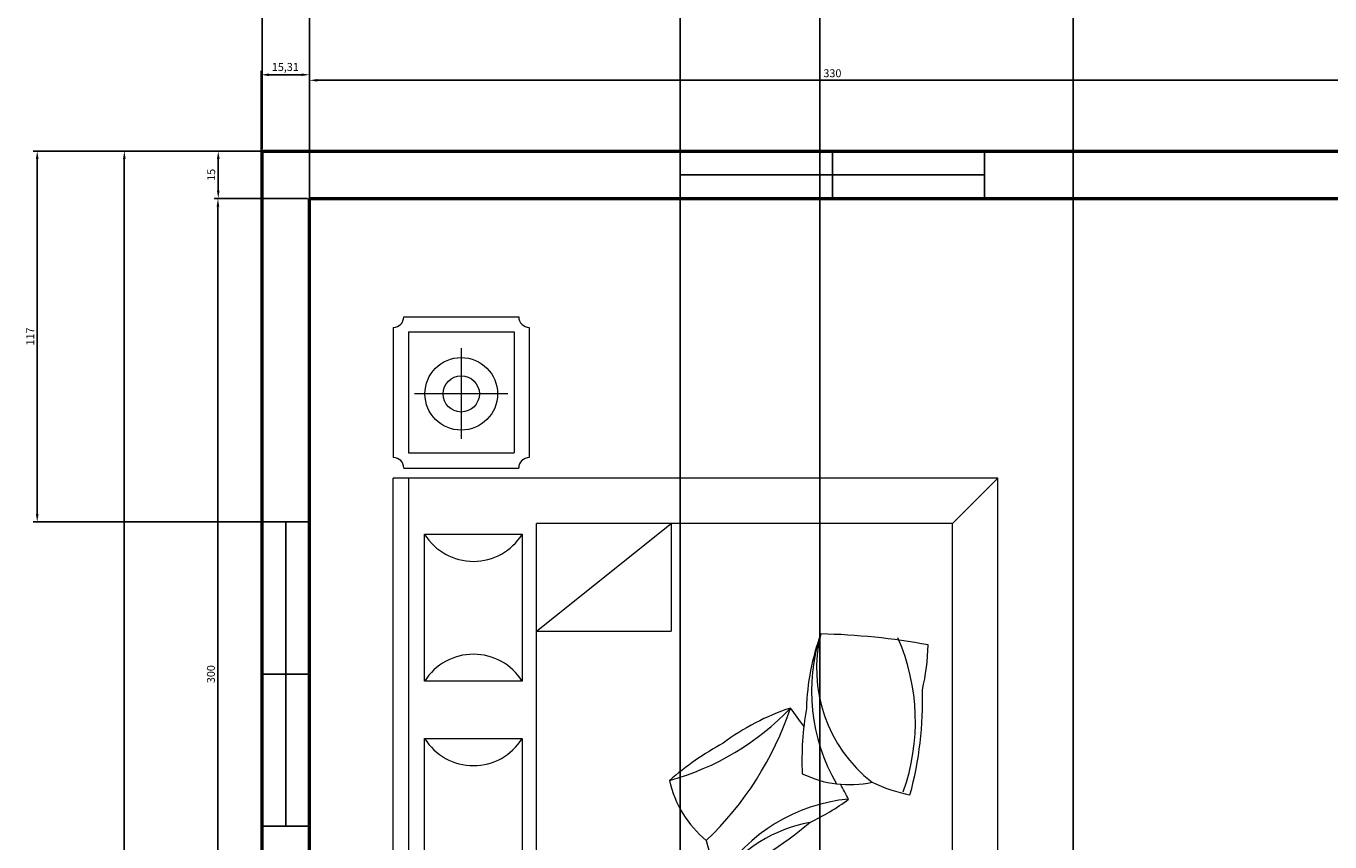
# Model space of a CAD drawing. Units: inches. Extents: x 604 to 3492, y -123 to 1737.
# Tile 14 of 20: x 1500 to 1912, y 1070 to 1327. Entities that reach past the tile are written whole.
import ezdxf

# ---------------------------------------------------------------- set-up
doc = ezdxf.new("R2010")
doc.units = ezdxf.units.IN
for name, color, linetype, lineweight in [('A-ANNO-DIMS', 2, 'Continuous', 18), ('A-FURN', 8, 'Continuous', 18), ('A-GLAZ', 4, 'Continuous', 25), ('A-WALL', 7, 'Continuous', 50)]:
    doc.layers.add(name, color=color, linetype=linetype, lineweight=lineweight)
doc.styles.get("Standard").update_dxf_attribs({"font": 'arial.ttf'})
doc.dimstyles.new('ISO-25', dxfattribs={"dimtxt": 2.5, "dimasz": 2.5, "dimexe": 1.25, "dimexo": 0.625, "dimtad": 1, "dimtxsty": 'Standard', "dimcen": 2.5, "dimadec": 0, "dimazin": 0, "dimtfac": 1, "dimtmove": 0, "dimatfit": 3, "dimfxl": 1, "dimarcsym": 0})

# ---------------------------------------------------------------- blocks, each defined once
blk = doc.blocks.new('A$C50B66110')
for p, q in [((0.0503, 1.9981), (0.4803, 1.9981)), ((0.1513, 1.6871), (0.1513, 1.9967)), ((0.5716, 1.9488), (0.5716, 2)), ((0.5716, 2), (2.0719, 2)), ((2.0719, 1.9488), (2.0719, 2)), ((2.5701, 1.9993), (2.1401, 1.9993)), ((0.0153, 1.9631), (0.0153, 1.5831)), ((0.0653, 1.9481), (0.0653, 1.5981)), ((0.0653, 1.9481), (0.4653, 1.9481)), ((0.4653, 1.9481), (0.4653, 1.5981)), ((0.5153, 1.9631), (0.5153, 1.5831)), ((2.0719, 1.9488), (0.5716, 1.9488)), ((0.5716, 1.9488), (0.5716, 0)), ((2.0719, 0), (2.0719, 1.9488)), ((2.1051, 1.9643), (2.1051, 1.5843)), ((2.1551, 1.9493), (2.1551, 1.5993)), ((2.5551, 1.9493), (2.1551, 1.9493)), ((2.5551, 1.9493), (2.5551, 1.5993)), ((2.6051, 1.9643), (2.6051, 1.5843)), ((2.3505, 1.62), (2.3505, 1.9295)), ((0.7257, 1.5725), (0.7257, 1.8954)), ((0.7257, 1.8954), (1.2113, 1.8954)), ((1.2113, 1.8954), (1.2113, 1.5725)), ((1.4007, 1.5725), (1.4007, 1.8954)), ((1.4007, 1.8954), (1.8863, 1.8954)), ((1.8863, 1.8954), (1.8863, 1.5725)), ((0, 1.8416), (0.2001, 1.8416)), ((2.5018, 1.7744), (2.2017, 1.7744)), ((0.0653, 1.5981), (0.4653, 1.5981)), ((2.5551, 1.5993), (2.1551, 1.5993)), ((1.2113, 1.5725), (0.7257, 1.5725)), ((1.8863, 1.5725), (1.4007, 1.5725)), ((0.0503, 1.5481), (0.4803, 1.5481)), ((1.5665, 1.5254), (1.5665, 1.0802)), ((1.5665, 1.5254), (1.9219, 1.0802)), ((2.5701, 1.5493), (2.1401, 1.5493)), ((1.9219, 1.0802), (1.5665, 1.0802)), ((0.5716, 0), (0.7216, 0.15)), ((2.0719, 0), (1.9219, 0.15)), ((0.5716, 0), (2.0719, 0))]:
    blk.add_line(p, q)
at = {"linetype": 'ByBlock'}
for p, q in [((0.2481, 1.9162), (0.2458, 1.9139)), ((0.2458, 1.9139), (0.2458, 1.7562)), ((0.2481, 1.9162), (0.4287, 1.9162)), ((0.2526, 1.9036), (0.2526, 1.8431)), ((0.3669, 1.9036), (0.2526, 1.9036)), ((0.3669, 1.8431), (0.3669, 1.9036)), ((0.3772, 1.9071), (0.3818, 1.9128)), ((0.3772, 1.7688), (0.3772, 1.9071)), ((0.3818, 1.9094), (0.3807, 1.9048)), ((0.3807, 1.9048), (0.3807, 1.8739)), ((0.3807, 1.9048), (0.3909, 1.8945)), ((0.3818, 1.9128), (0.4161, 1.9128)), ((0.3864, 1.9116), (0.3818, 1.9094)), ((0.3921, 1.8968), (0.3864, 1.9116)), ((0.3864, 1.9116), (0.4138, 1.9116)), ((0.4081, 1.8968), (0.4138, 1.9116)), ((0.4195, 1.9048), (0.4092, 1.8945)), ((0.4138, 1.9116), (0.4184, 1.9094)), ((0.4161, 1.9128), (0.4218, 1.9071)), ((0.4184, 1.9094), (0.4195, 1.9048)), ((0.4195, 1.9048), (0.4195, 1.8739)), ((0.4218, 1.9071), (0.4218, 1.7699)), ((0.4287, 1.9162), (0.4309, 1.9139)), ((0.4309, 1.9139), (0.4309, 1.7562)), ((0.3807, 1.8739), (0.3829, 1.8682)), ((0.3829, 1.8682), (0.3864, 1.8625)), ((0.3864, 1.8625), (0.3875, 1.8545)), ((0.3875, 1.8545), (0.3875, 1.8431)), ((0.3909, 1.8945), (0.3921, 1.8968)), ((0.3909, 1.8431), (0.3909, 1.8945)), ((0.4081, 1.8968), (0.3921, 1.8968)), ((0.4092, 1.8945), (0.4081, 1.8968)), ((0.4092, 1.8431), (0.4092, 1.8945)), ((0.4138, 1.8625), (0.4127, 1.8545)), ((0.4127, 1.8545), (0.4127, 1.8431)), ((0.4172, 1.8682), (0.4138, 1.8625)), ((0.4195, 1.8739), (0.4172, 1.8682)), ((0.2526, 1.8431), (0.3669, 1.8431)), ((0.3201, 1.8168), (0.2526, 1.8168)), ((0.2526, 1.8168), (0.2526, 1.7962)), ((0.2572, 1.8408), (0.2572, 1.8294)), ((0.3669, 1.8408), (0.2572, 1.8408)), ((0.2572, 1.8294), (0.3669, 1.8294)), ((0.2675, 1.8145), (0.2641, 1.8145)), ((0.2641, 1.8145), (0.2641, 1.8111)), ((0.2641, 1.8111), (0.2675, 1.8111)), ((0.2664, 1.8408), (0.2664, 1.8294)), ((0.2675, 1.8111), (0.2675, 1.8145)), ((0.2755, 1.8408), (0.2755, 1.8294)), ((0.2846, 1.8408), (0.2846, 1.8294)), ((0.2846, 1.8145), (0.2846, 1.8111)), ((0.2881, 1.8145), (0.2846, 1.8145)), ((0.2846, 1.8111), (0.2881, 1.8111)), ((0.2881, 1.8111), (0.2881, 1.8145)), ((0.2938, 1.8408), (0.2938, 1.8294)), ((0.3029, 1.8408), (0.3029, 1.8294)), ((0.3052, 1.8145), (0.3052, 1.8111)), ((0.3086, 1.8145), (0.3052, 1.8145)), ((0.3052, 1.8111), (0.3086, 1.8111)), ((0.3086, 1.8111), (0.3086, 1.8145)), ((0.3121, 1.8408), (0.3121, 1.8294)), ((0.3201, 1.7962), (0.3201, 1.8168)), ((0.3304, 1.8111), (0.3395, 1.8111)), ((0.3304, 1.8042), (0.3304, 1.8111)), ((0.3395, 1.8111), (0.3395, 1.8042)), ((0.3441, 1.8042), (0.3441, 1.8111)), ((0.3441, 1.8111), (0.3532, 1.8111)), ((0.3532, 1.8111), (0.3532, 1.8042)), ((0.3578, 1.8111), (0.3669, 1.8111)), ((0.3578, 1.8042), (0.3578, 1.8111)), ((0.3669, 1.8294), (0.3669, 1.8408)), ((0.3669, 1.8111), (0.3669, 1.8042)), ((0.3829, 1.8076), (0.3864, 1.8134)), ((0.3864, 1.8134), (0.3875, 1.8214)), ((0.3875, 1.8214), (0.3875, 1.8431)), ((0.3909, 1.8431), (0.3909, 1.7813)), ((0.4092, 1.8431), (0.4092, 1.7813)), ((0.4127, 1.8214), (0.4127, 1.8431)), ((0.4138, 1.8134), (0.4127, 1.8214)), ((0.4172, 1.8076), (0.4138, 1.8134)), ((0.2526, 1.7962), (0.3201, 1.7962)), ((0.2652, 1.7905), (0.2538, 1.7905)), ((0.2538, 1.7905), (0.2538, 1.7859)), ((0.2538, 1.7859), (0.2652, 1.7859)), ((0.2538, 1.7665), (0.2538, 1.7733)), ((0.2538, 1.7733), (0.2652, 1.7733)), ((0.2641, 1.8019), (0.2641, 1.7985)), ((0.2675, 1.8019), (0.2641, 1.8019)), ((0.2641, 1.7985), (0.2675, 1.7985)), ((0.2652, 1.7859), (0.2652, 1.7905)), ((0.2652, 1.7733), (0.2652, 1.7665)), ((0.2675, 1.7985), (0.2675, 1.8019)), ((0.2812, 1.7905), (0.2698, 1.7905)), ((0.2698, 1.7905), (0.2698, 1.7859)), ((0.2698, 1.7859), (0.2812, 1.7859)), ((0.2698, 1.7665), (0.2698, 1.7733)), ((0.2698, 1.7733), (0.2812, 1.7733)), ((0.2812, 1.7859), (0.2812, 1.7905)), ((0.2812, 1.7733), (0.2812, 1.7665)), ((0.2846, 1.8019), (0.2846, 1.7985)), ((0.2881, 1.8019), (0.2846, 1.8019)), ((0.2846, 1.7985), (0.2881, 1.7985)), ((0.2972, 1.7905), (0.2858, 1.7905)), ((0.2858, 1.7905), (0.2858, 1.7859)), ((0.2858, 1.7859), (0.2972, 1.7859)), ((0.2858, 1.7665), (0.2858, 1.7733)), ((0.2858, 1.7733), (0.2972, 1.7733)), ((0.2881, 1.7985), (0.2881, 1.8019)), ((0.2972, 1.7859), (0.2972, 1.7905)), ((0.2972, 1.7733), (0.2972, 1.7665)), ((0.3018, 1.7905), (0.3018, 1.7859)), ((0.3132, 1.7905), (0.3018, 1.7905)), ((0.3018, 1.7859), (0.3132, 1.7859)), ((0.3018, 1.7733), (0.3132, 1.7733)), ((0.3018, 1.7665), (0.3018, 1.7733)), ((0.3052, 1.8019), (0.3052, 1.7985)), ((0.3086, 1.8019), (0.3052, 1.8019)), ((0.3052, 1.7985), (0.3086, 1.7985)), ((0.3086, 1.7985), (0.3086, 1.8019)), ((0.3132, 1.7859), (0.3132, 1.7905)), ((0.3132, 1.7733), (0.3132, 1.7665)), ((0.3395, 1.8042), (0.3304, 1.8042)), ((0.3304, 1.7985), (0.3395, 1.7985)), ((0.3304, 1.7916), (0.3304, 1.7985)), ((0.3395, 1.7916), (0.3304, 1.7916)), ((0.3304, 1.7779), (0.3304, 1.7848)), ((0.3304, 1.7848), (0.3395, 1.7848)), ((0.3395, 1.7779), (0.3304, 1.7779)), ((0.3304, 1.7722), (0.3395, 1.7722)), ((0.3304, 1.7653), (0.3304, 1.7722)), ((0.3395, 1.7985), (0.3395, 1.7916)), ((0.3395, 1.7848), (0.3395, 1.7779)), ((0.3395, 1.7722), (0.3395, 1.7653)), ((0.3532, 1.8042), (0.3441, 1.8042)), ((0.3441, 1.7985), (0.3532, 1.7985)), ((0.3441, 1.7916), (0.3441, 1.7985)), ((0.3532, 1.7916), (0.3441, 1.7916)), ((0.3441, 1.7779), (0.3441, 1.7848)), ((0.3441, 1.7848), (0.3532, 1.7848)), ((0.3532, 1.7779), (0.3441, 1.7779)), ((0.3441, 1.7722), (0.3532, 1.7722)), ((0.3441, 1.7653), (0.3441, 1.7722)), ((0.3532, 1.7985), (0.3532, 1.7916)), ((0.3532, 1.7848), (0.3532, 1.7779)), ((0.3532, 1.7722), (0.3532, 1.7653)), ((0.3669, 1.8042), (0.3578, 1.8042)), ((0.3578, 1.7985), (0.3669, 1.7985)), ((0.3578, 1.7916), (0.3578, 1.7985)), ((0.3669, 1.7916), (0.3578, 1.7916)), ((0.3578, 1.7791), (0.3578, 1.7859)), ((0.3578, 1.7859), (0.3669, 1.7859)), ((0.3669, 1.7791), (0.3578, 1.7791)), ((0.3578, 1.7653), (0.3578, 1.7722)), ((0.3578, 1.7722), (0.3669, 1.7722)), ((0.3669, 1.7985), (0.3669, 1.7916)), ((0.3669, 1.7859), (0.3669, 1.7791)), ((0.3669, 1.7722), (0.3669, 1.7653)), ((0.3829, 1.7631), (0.3772, 1.7688)), ((0.3807, 1.8019), (0.3829, 1.8076)), ((0.3807, 1.7711), (0.3807, 1.8019)), ((0.3807, 1.7711), (0.3909, 1.7813)), ((0.3818, 1.7665), (0.3807, 1.7711)), ((0.3921, 1.7791), (0.3864, 1.7642)), ((0.3909, 1.7813), (0.3921, 1.7791)), ((0.4081, 1.7791), (0.3921, 1.7791)), ((0.4092, 1.7813), (0.4081, 1.7791)), ((0.4081, 1.7791), (0.4138, 1.7642)), ((0.4195, 1.7711), (0.4092, 1.7813)), ((0.4218, 1.7699), (0.4161, 1.7631)), ((0.4195, 1.8019), (0.4172, 1.8076)), ((0.4184, 1.7665), (0.4195, 1.7711)), ((0.4195, 1.7711), (0.4195, 1.8019)), ((0.4378, 1.7742), (0.4309, 1.7768)), ((0.4309, 1.7722), (0.436, 1.7708)), ((0.436, 1.7708), (0.4406, 1.7672)), ((0.441, 1.771), (0.4378, 1.7742)), ((0.4434, 1.7688), (0.441, 1.771)), ((0.4477, 1.7704), (0.4434, 1.7688)), ((0.4497, 1.7684), (0.4477, 1.7704)), ((0.4481, 1.765), (0.4497, 1.7684)), ((0.2458, 1.7562), (0.2481, 1.7539)), ((0.4, 1.7539), (0.2481, 1.7539)), ((0.2652, 1.7665), (0.2538, 1.7665)), ((0.2812, 1.7665), (0.2698, 1.7665)), ((0.2972, 1.7665), (0.2858, 1.7665)), ((0.3132, 1.7665), (0.3018, 1.7665)), ((0.3395, 1.7653), (0.3304, 1.7653)), ((0.3532, 1.7653), (0.3441, 1.7653)), ((0.3669, 1.7653), (0.3578, 1.7653)), ((0.3864, 1.7642), (0.3818, 1.7665)), ((0.399, 1.7631), (0.3829, 1.7631)), ((0.3864, 1.7642), (0.399, 1.7642)), ((0.4024, 1.7676), (0.3989, 1.7676)), ((0.3989, 1.7676), (0.3991, 1.7578)), ((0.3991, 1.7578), (0.4019, 1.7462)), ((0.4019, 1.7462), (0.4047, 1.7353)), ((0.4026, 1.7254), (0.4021, 1.7198)), ((0.403, 1.7585), (0.4024, 1.7676)), ((0.4026, 1.7642), (0.4138, 1.7642)), ((0.4051, 1.7279), (0.4026, 1.7254)), ((0.4161, 1.7631), (0.4027, 1.7631)), ((0.4047, 1.7511), (0.403, 1.7585)), ((0.4287, 1.7539), (0.404, 1.7539)), ((0.4047, 1.7353), (0.4044, 1.7293)), ((0.4044, 1.7293), (0.4051, 1.7279)), ((0.4074, 1.7402), (0.4047, 1.7511)), ((0.4081, 1.7346), (0.4074, 1.7402)), ((0.4079, 1.7286), (0.4081, 1.7346)), ((0.4121, 1.7256), (0.4079, 1.7286)), ((0.4111, 1.7203), (0.4121, 1.7256)), ((0.4138, 1.7642), (0.4184, 1.7665)), ((0.4309, 1.7562), (0.4287, 1.7539)), ((0.4406, 1.7672), (0.4418, 1.7656)), ((0.4443, 1.7658), (0.4418, 1.7633)), ((0.4418, 1.7656), (0.4443, 1.7658)), ((0.4418, 1.7633), (0.4511, 1.7551)), ((0.4509, 1.7672), (0.4481, 1.765)), ((0.4539, 1.764), (0.4509, 1.7672)), ((0.4511, 1.7551), (0.4662, 1.7422)), ((0.4515, 1.7573), (0.4539, 1.764)), ((0.4577, 1.7605), (0.4515, 1.7573)), ((0.463, 1.7555), (0.4577, 1.7605)), ((0.4618, 1.7482), (0.463, 1.7555)), ((0.467, 1.7515), (0.4618, 1.7482)), ((0.4664, 1.7418), (0.4741, 1.72)), ((0.4714, 1.7468), (0.467, 1.7515)), ((0.4696, 1.7418), (0.4714, 1.7468)), ((0.4766, 1.7425), (0.4697, 1.7418)), ((0.472, 1.733), (0.4787, 1.7356)), ((0.4794, 1.7332), (0.472, 1.733)), ((0.4761, 1.7233), (0.481, 1.7279)), ((0.4787, 1.7356), (0.4766, 1.7425)), ((0.481, 1.7279), (0.4794, 1.7332)), ((0.4021, 1.7198), (0.4088, 1.7187)), ((0.4088, 1.7187), (0.4023, 1.7147)), ((0.4023, 1.7147), (0.4028, 1.7085)), ((0.4028, 1.7085), (0.4102, 1.7078)), ((0.4102, 1.7078), (0.4037, 1.7027)), ((0.4037, 1.7027), (0.4067, 1.6974)), ((0.4067, 1.6974), (0.4137, 1.6988)), ((0.4137, 1.6988), (0.4104, 1.6923)), ((0.4104, 1.6923), (0.4139, 1.6881)), ((0.4123, 1.7057), (0.4111, 1.7203)), ((0.4211, 1.6946), (0.4123, 1.7057)), ((0.4139, 1.6881), (0.4192, 1.692)), ((0.4192, 1.692), (0.4183, 1.6858)), ((0.4183, 1.6858), (0.4227, 1.683)), ((0.4333, 1.6881), (0.4211, 1.6946)), ((0.4227, 1.683), (0.4283, 1.6876)), ((0.4283, 1.6876), (0.4276, 1.68)), ((0.4324, 1.6786), (0.4354, 1.6849)), ((0.4472, 1.6869), (0.4333, 1.6881)), ((0.4354, 1.6849), (0.4382, 1.6786)), ((0.4421, 1.6782), (0.4437, 1.6849)), ((0.4437, 1.6849), (0.4463, 1.6775)), ((0.4606, 1.6927), (0.4472, 1.6869)), ((0.4507, 1.6786), (0.4509, 1.6849)), ((0.4509, 1.6849), (0.4562, 1.6802)), ((0.4562, 1.6802), (0.4599, 1.6821)), ((0.4592, 1.689), (0.4641, 1.683)), ((0.4599, 1.6821), (0.4592, 1.689)), ((0.4708, 1.7027), (0.4606, 1.6927)), ((0.4641, 1.683), (0.4678, 1.6863)), ((0.465, 1.6925), (0.4715, 1.6897)), ((0.4678, 1.6863), (0.465, 1.6925)), ((0.4741, 1.72), (0.4708, 1.7027)), ((0.4745, 1.6925), (0.4713, 1.6988)), ((0.4713, 1.6988), (0.478, 1.6967)), ((0.4715, 1.6897), (0.4745, 1.6925)), ((0.4743, 1.7075), (0.4815, 1.7073)), ((0.4798, 1.7013), (0.4743, 1.7075)), ((0.4824, 1.7233), (0.4761, 1.7233)), ((0.4764, 1.7154), (0.4835, 1.7175)), ((0.4824, 1.7119), (0.4764, 1.7154)), ((0.478, 1.6967), (0.4798, 1.7013)), ((0.4815, 1.7073), (0.4824, 1.7119)), ((0.4835, 1.7175), (0.4824, 1.7233)), ((0.4276, 1.68), (0.4324, 1.6786)), ((0.4382, 1.6786), (0.4421, 1.6782)), ((0.4463, 1.6775), (0.4507, 1.6786)), ((0.7216, 1.5254), (1.9219, 1.5254)), ((0.7216, 1.5254), (0.7216, 0.15)), ((1.9219, 0.15), (1.9219, 1.5254)), ((0.7216, 0.15), (1.9219, 0.15))]:
    blk.add_line(p, q, dxfattribs=at)
for centre, radius in [((0.1513, 1.8416), 0.12), ((0.1513, 1.8416), 0.06), ((2.3505, 1.7744), 0.12), ((2.3505, 1.7744), 0.06)]:
    blk.add_circle(centre, radius)
for centre, radius, start, end in [((0.0153, 1.9981), 0.035, 270, 0), ((0.5153, 1.9981), 0.035, 180, 270), ((2.1051, 1.9993), 0.035, 270, 0), ((2.6051, 1.9993), 0.035, 180, 270), ((0.6244, 1.734), 0.1906, 302.1202, 57.8798), ((1.3126, 1.734), 0.1906, 122.1202, 237.8798), ((1.2994, 1.734), 0.1906, 302.1202, 57.8798), ((1.9876, 1.734), 0.1906, 122.1202, 237.8798), ((0.0153, 1.5481), 0.035, 0, 90), ((0.5153, 1.5481), 0.035, 90, 180), ((2.1051, 1.5493), 0.035, 0, 90), ((2.6051, 1.5493), 0.035, 90, 180), ((1.1502, 0.7366), 0.3575, 102.4782, 140.4625), ((0.328, 0.4368), 0.9879, 28.4971, 41.0566), ((1.9117, 1.3157), 0.8697, 195.336, 226.4193), ((0.9996, 0.4307), 0.548, 103.2034, 117.0362), ((1.656, 1.7093), 1.0798, 223.6306, 251.4288), ((0.4482, 0.4408), 0.5655, 5.3391, 57.6895), ((1.8226, 1.3753), 1.1652, 203.0642, 220.3209), ((0.4548, 0.5307), 0.4879, 10.6986, 52.6864), ((0.5648, 0.4378), 0.7874, 18.3527, 36.6851), ((1.4166, 0.4903), 0.3575, 154.0418, 192.0262), ((1.1403, -0.3401), 0.9879, 80.0607, 92.6202), ((-0.0179, 2.4352), 2.1977, 305.2966, 307.2418), ((1.5981, 0.9345), 0.734, 205.259, 216.9351), ((1.3672, 0.0075), 0.6085, 71.81, 120.1351), ((1.2867, -0.154), 0.7874, 69.9163, 88.2487), ((1.4431, 0.1219), 0.4774, 76.1849, 142.0017), ((-0.6401, 0.6314), 2.1977, 349.4884, 358.8054), ((-0.0179, 2.4352), 2.1977, 297.9248, 299.3793), ((1.5626, 0.1822), 0.548, 154.767, 168.5998), ((1.2678, 0.9611), 0.6885, 250.2936, 293.6414), ((1.3343, 1.4141), 1.1652, 254.6278, 271.8845), ((1.5399, 0.9642), 0.734, 256.8226, 268.4988)]:
    blk.add_arc(centre, radius, start, end)
blk = doc.blocks.new('*D38')
at = {"layer": 'A-ANNO-DIMS', "color": 0, "lineweight": -2, "transparency": 16777216}
for p, q in [((1574.26, 1273.33), (1574.26, 1313.01)), ((1589.57, 1273.33), (1589.57, 1313.01)), ((1587.07, 1311.76), (1576.76, 1311.76))]:
    blk.add_line(p, q, dxfattribs=at)
at = {"layer": 'A-ANNO-DIMS', "color": 0, "transparency": 16777216}
for points in [[(1576.76, 1312.18), (1576.76, 1311.34), (1574.26, 1311.76)], [(1587.07, 1312.18), (1587.07, 1311.34), (1589.57, 1311.76)]]:
    blk.add_solid(points, dxfattribs=at)
at = {"layer": 'Defpoints', "color": 0, "transparency": 16777216}
for p in [(1574.26, 1311.76), (1574.26, 1272.7), (1589.57, 1272.7)]:
    blk.add_point(p, dxfattribs=at)
at = {"layer": 'A-ANNO-DIMS', "color": 0, "transparency": 16777216, "insert": (1581.92, 1313.89), "char_height": 2.5, "attachment_point": 5}
blk.add_mtext('15,31', dxfattribs=at)
blk = doc.blocks.new('*D39')
at = {"layer": 'A-ANNO-DIMS', "color": 0, "lineweight": -2, "transparency": 16777216}
for p, q in [((1589.57, 1273.33), (1589.57, 1311.26)), ((1592.07, 1310.01), (1917.07, 1310.01)), ((1919.57, 1273.33), (1919.57, 1311.26))]:
    blk.add_line(p, q, dxfattribs=at)
at = {"layer": 'A-ANNO-DIMS', "color": 0, "transparency": 16777216}
for points in [[(1592.07, 1310.43), (1592.07, 1309.59), (1589.57, 1310.01)], [(1917.07, 1310.43), (1917.07, 1309.59), (1919.57, 1310.01)]]:
    blk.add_solid(points, dxfattribs=at)
at = {"layer": 'Defpoints', "color": 0, "transparency": 16777216}
for p in [(1919.57, 1310.01), (1589.57, 1272.7), (1919.57, 1272.7)]:
    blk.add_point(p, dxfattribs=at)
at = {"layer": 'A-ANNO-DIMS', "color": 0, "transparency": 16777216, "insert": (1754.57, 1311.91), "char_height": 2.5, "attachment_point": 5}
blk.add_mtext('330', dxfattribs=at)
blk = doc.blocks.new('*D60')
at = {"layer": 'A-ANNO-DIMS', "color": 0, "lineweight": -2, "transparency": 16777216}
for p, q in [((1588.95, 1287.7), (1559.5, 1287.7)), ((1560.75, 1285.2), (1560.75, 1275.2)), ((1588.95, 1272.7), (1559.5, 1272.7))]:
    blk.add_line(p, q, dxfattribs=at)
at = {"layer": 'A-ANNO-DIMS', "color": 0, "transparency": 16777216}
for points in [[(1560.34, 1285.2), (1561.17, 1285.2), (1560.75, 1287.7)], [(1560.34, 1275.2), (1561.17, 1275.2), (1560.75, 1272.7)]]:
    blk.add_solid(points, dxfattribs=at)
at = {"layer": 'Defpoints', "color": 0, "transparency": 16777216}
for p in [(1589.57, 1287.7), (1560.75, 1272.7), (1589.57, 1272.7)]:
    blk.add_point(p, dxfattribs=at)
at = {"layer": 'A-ANNO-DIMS', "color": 0, "transparency": 16777216, "insert": (1558.85, 1280.2), "char_height": 2.5, "attachment_point": 5, "rotation": 90}
blk.add_mtext('15', dxfattribs=at)
blk = doc.blocks.new('*D61')
at = {"layer": 'A-ANNO-DIMS', "color": 0, "lineweight": -2, "transparency": 16777216}
for p, q in [((1588.95, 1272.7), (1559.41, 1272.7)), ((1560.66, 1270.2), (1560.66, 975.2)), ((1588.95, 972.7), (1559.41, 972.7))]:
    blk.add_line(p, q, dxfattribs=at)
at = {"layer": 'A-ANNO-DIMS', "color": 0, "transparency": 16777216}
for points in [[(1560.24, 1270.2), (1561.07, 1270.2), (1560.66, 1272.7)], [(1560.24, 975.2), (1561.07, 975.2), (1560.66, 972.7)]]:
    blk.add_solid(points, dxfattribs=at)
at = {"layer": 'Defpoints', "color": 0, "transparency": 16777216}
for p in [(1589.57, 1272.7), (1560.66, 972.7), (1589.57, 972.7)]:
    blk.add_point(p, dxfattribs=at)
at = {"layer": 'A-ANNO-DIMS', "color": 0, "transparency": 16777216, "insert": (1558.76, 1122.7), "char_height": 2.5, "attachment_point": 5, "rotation": 90}
blk.add_mtext('300', dxfattribs=at)
blk = doc.blocks.new('*D69')
at = {"layer": 'A-ANNO-DIMS', "color": 0, "lineweight": -2, "transparency": 16777216}
for p, q in [((1573.95, 1287.7), (1529.86, 1287.7)), ((1531.11, 290.2), (1531.11, 1285.2)), ((1573.95, 287.7), (1529.86, 287.7))]:
    blk.add_line(p, q, dxfattribs=at)
at = {"layer": 'A-ANNO-DIMS', "color": 0, "transparency": 16777216}
for points in [[(1530.69, 1285.2), (1531.52, 1285.2), (1531.11, 1287.7)], [(1530.69, 290.2), (1531.52, 290.2), (1531.11, 287.7)]]:
    blk.add_solid(points, dxfattribs=at)
at = {"layer": 'Defpoints', "color": 0, "transparency": 16777216}
for p in [(1531.11, 1287.7), (1574.57, 1287.7), (1574.57, 287.7)]:
    blk.add_point(p, dxfattribs=at)
at = {"layer": 'A-ANNO-DIMS', "color": 0, "transparency": 16777216, "insert": (1529.21, 787.7), "char_height": 2.5, "attachment_point": 5, "rotation": 90}
blk.add_mtext('1000', dxfattribs=at)
blk = doc.blocks.new('*D71')
at = {"layer": 'A-ANNO-DIMS', "color": 0, "lineweight": -2, "transparency": 16777216}
for p, q in [((1574.57, 1288.33), (1574.57, 1357.82)), ((1577.07, 1356.57), (2247.07, 1356.57)), ((2249.57, 1288.33), (2249.57, 1357.82))]:
    blk.add_line(p, q, dxfattribs=at)
at = {"layer": 'A-ANNO-DIMS', "color": 0, "transparency": 16777216}
for points in [[(1577.07, 1356.98), (1577.07, 1356.15), (1574.57, 1356.57)], [(2247.07, 1356.98), (2247.07, 1356.15), (2249.57, 1356.57)]]:
    blk.add_solid(points, dxfattribs=at)
at = {"layer": 'Defpoints', "color": 0, "transparency": 16777216}
for p in [(2249.57, 1356.57), (1574.57, 1287.7), (2249.57, 1287.7)]:
    blk.add_point(p, dxfattribs=at)
at = {"layer": 'A-ANNO-DIMS', "color": 0, "transparency": 16777216, "insert": (1912.07, 1358.47), "char_height": 2.5, "attachment_point": 5}
blk.add_mtext('675', dxfattribs=at)
blk = doc.blocks.new('WIN-96')
for p, q in [((15, 96), (0, 96)), ((7.5, 96), (7.5, 0)), ((15, 96), (15, 0)), ((15, 48), (0, 48))]:
    blk.add_line(p, q)
blk.add_lwpolyline([(0, 96), (0, 0), (15, 0), (15, 96)], close=True)
blk = doc.blocks.new('*D100')
at = {"layer": 'A-ANNO-DIMS', "color": 0, "lineweight": -2, "transparency": 16777216}
for p, q in [((1589.57, 843.33), (1589.57, 1359.9)), ((1592.07, 1358.65), (1828.07, 1358.65)), ((1830.57, 843.33), (1830.57, 1359.9))]:
    blk.add_line(p, q, dxfattribs=at)
at = {"layer": 'A-ANNO-DIMS', "color": 0, "transparency": 16777216}
for points in [[(1592.07, 1359.07), (1592.07, 1358.23), (1589.57, 1358.65)], [(1828.07, 1359.07), (1828.07, 1358.23), (1830.57, 1358.65)]]:
    blk.add_solid(points, dxfattribs=at)
at = {"layer": 'Defpoints', "color": 0, "transparency": 16777216}
for p in [(1830.57, 1358.65), (1589.57, 842.7), (1830.57, 842.7)]:
    blk.add_point(p, dxfattribs=at)
at = {"layer": 'A-ANNO-DIMS', "color": 0, "transparency": 16777216, "insert": (1710.07, 1360.53), "char_height": 2.5, "attachment_point": 5}
blk.add_mtext('241', dxfattribs=at)
blk = doc.blocks.new('*D103')
at = {"layer": 'A-ANNO-DIMS', "color": 0, "lineweight": -2, "transparency": 16777216}
for p, q in [((1589.57, 1272.08), (1589.57, 215.5)), ((1706.57, 1272.08), (1706.57, 215.5)), ((1592.07, 216.75), (1704.07, 216.75))]:
    blk.add_line(p, q, dxfattribs=at)
at = {"layer": 'A-ANNO-DIMS', "color": 0, "transparency": 16777216}
for points in [[(1592.07, 217.17), (1592.07, 216.33), (1589.57, 216.75)], [(1704.07, 217.17), (1704.07, 216.33), (1706.57, 216.75)]]:
    blk.add_solid(points, dxfattribs=at)
at = {"layer": 'Defpoints', "color": 0, "transparency": 16777216}
for p in [(1589.57, 1272.7), (1706.57, 1272.7), (1706.57, 216.75)]:
    blk.add_point(p, dxfattribs=at)
at = {"layer": 'A-ANNO-DIMS', "color": 0, "transparency": 16777216, "insert": (1648.07, 218.63), "char_height": 2.5, "attachment_point": 5}
blk.add_mtext('117', dxfattribs=at)
blk = doc.blocks.new('*D105')
at = {"layer": 'A-ANNO-DIMS', "color": 0, "lineweight": -2, "transparency": 16777216}
for p, q in [((1573.95, 1287.7), (1502.37, 1287.7)), ((1503.62, 1173.2), (1503.62, 1285.2)), ((1573.95, 1170.7), (1502.37, 1170.7))]:
    blk.add_line(p, q, dxfattribs=at)
at = {"layer": 'A-ANNO-DIMS', "color": 0, "transparency": 16777216}
for points in [[(1503.21, 1285.2), (1504.04, 1285.2), (1503.62, 1287.7)], [(1503.21, 1173.2), (1504.04, 1173.2), (1503.62, 1170.7)]]:
    blk.add_solid(points, dxfattribs=at)
at = {"layer": 'Defpoints', "color": 0, "transparency": 16777216}
for p in [(1503.62, 1287.7), (1574.57, 1287.7), (1574.57, 1170.7)]:
    blk.add_point(p, dxfattribs=at)
at = {"layer": 'A-ANNO-DIMS', "color": 0, "transparency": 16777216, "insert": (1501.74, 1229.2), "char_height": 2.5, "attachment_point": 5, "rotation": 90}
blk.add_mtext('117', dxfattribs=at)
blk = doc.blocks.new('*D108')
at = {"layer": 'A-ANNO-DIMS', "color": 0, "lineweight": -2, "transparency": 16777216}
for p, q in [((1589.57, 303.33), (1589.57, 1359.9)), ((1592.07, 1358.65), (1704.07, 1358.65)), ((1706.57, 303.33), (1706.57, 1359.9))]:
    blk.add_line(p, q, dxfattribs=at)
at = {"layer": 'A-ANNO-DIMS', "color": 0, "transparency": 16777216}
for points in [[(1592.07, 1359.07), (1592.07, 1358.23), (1589.57, 1358.65)], [(1704.07, 1359.07), (1704.07, 1358.23), (1706.57, 1358.65)]]:
    blk.add_solid(points, dxfattribs=at)
at = {"layer": 'Defpoints', "color": 0, "transparency": 16777216}
for p in [(1706.57, 1358.65), (1589.57, 302.7), (1706.57, 302.7)]:
    blk.add_point(p, dxfattribs=at)
at = {"layer": 'A-ANNO-DIMS', "color": 0, "transparency": 16777216, "insert": (1648.07, 1360.53), "char_height": 2.5, "attachment_point": 5}
blk.add_mtext('117', dxfattribs=at)
blk = doc.blocks.new('*D110')
at = {"layer": 'A-ANNO-DIMS', "color": 0, "lineweight": -2, "transparency": 16777216}
for p, q in [((1589.57, 973.33), (1589.57, 1359.9)), ((1592.07, 1358.65), (1748.07, 1358.65)), ((1750.57, 973.33), (1750.57, 1359.9))]:
    blk.add_line(p, q, dxfattribs=at)
at = {"layer": 'A-ANNO-DIMS', "color": 0, "transparency": 16777216}
for points in [[(1592.07, 1359.07), (1592.07, 1358.23), (1589.57, 1358.65)], [(1748.07, 1359.07), (1748.07, 1358.23), (1750.57, 1358.65)]]:
    blk.add_solid(points, dxfattribs=at)
at = {"layer": 'Defpoints', "color": 0, "transparency": 16777216}
for p in [(1750.57, 1358.65), (1589.57, 972.7), (1750.57, 972.7)]:
    blk.add_point(p, dxfattribs=at)
at = {"layer": 'A-ANNO-DIMS', "color": 0, "transparency": 16777216, "insert": (1670.07, 1360.55), "char_height": 2.5, "attachment_point": 5}
blk.add_mtext('161', dxfattribs=at)

msp = doc.modelspace()

# ---------------------------------------------------------------- linework, layer by layer
at = {"layer": 'A-WALL'}
for p, q in [((1574.5743, 1287.7004), (2249.5743, 1287.7004)), ((1574.5743, 287.7004), (1574.5743, 1287.7004)), ((1589.5743, 1272.7004), (1919.5743, 1272.7004)), ((1589.5743, 1272.7004), (1919.5743, 1272.7004)), ((1589.5743, 972.7004), (1589.5743, 1272.7004)), ((1589.5743, 972.7004), (1589.5743, 1272.7004))]:
    msp.add_line(p, q, dxfattribs=at)

# ---------------------------------------------------------------- block references
at = {"layer": 'A-FURN', "xscale": 95.4379570199766, "yscale": 95.4379570199766, "zscale": 95.4379570199766, "rotation": 90}
msp.add_blockref('A$C50B66110', (1806.779, 986.7784), dxfattribs=at)
at = {"layer": 'A-GLAZ', "rotation": 89.99999999999909}
msp.add_blockref('WIN-96', (1802.5743, 1272.7004), dxfattribs=at)
at = {"layer": 'A-GLAZ'}
msp.add_blockref('WIN-96', (1574.5743, 1074.7004), dxfattribs=at)

# ---------------------------------------------------------------- dimensions: what is measured, and where the dimension line sits
at = {"layer": 'A-ANNO-DIMS'}
for base, p1, p2, override, picture, middle in [((1750.5743, 1358.6504), (1589.5743, 972.7004), (1750.5743, 972.7004), {"dimdec": 0, "dimlfac": 1, "dimrnd": 0, "dimzin": 0, "dimdsep": 46, "dimlunit": 2}, '*D110', (1670.0743, 1360.5519)), ((1830.5743, 1358.6504), (1589.5743, 842.7004), (1830.5743, 842.7004), {"dimdec": 0, "dimlfac": 1, "dimrnd": 0, "dimzin": 0, "dimdsep": 46, "dimlunit": 2}, '*D100', (1710.0743, 1360.5306)), ((1706.5743, 1358.6504), (1589.5743, 302.7004), (1706.5743, 302.7004), {"dimdec": 0, "dimlfac": 1, "dimrnd": 0, "dimzin": 0, "dimdsep": 46, "dimlunit": 2}, '*D108', (1648.0743, 1360.5306)), ((1574.2644, 1311.7593), (1589.5743, 1272.7004), (1574.2644, 1272.7004), {"dimclrd": 0, "dimclre": 0, "dimclrt": 0}, '*D38', (1581.9194, 1313.8867)), ((1919.5743, 1310.0107), (1589.5743, 1272.7004), (1919.5743, 1272.7004), {"dimclrd": 0, "dimclre": 0, "dimclrt": 0}, '*D39', (1754.5743, 1311.913)), ((1706.5743, 216.7504), (1589.5743, 1272.7004), (1706.5743, 1272.7004), {"dimdec": 0, "dimlfac": 1, "dimrnd": 0, "dimzin": 0, "dimdsep": 46, "dimlunit": 2}, '*D103', (1648.0743, 218.6306))]:
    dim = msp.add_linear_dim(base=base, p1=p1, p2=p2, dimstyle='ISO-25', override=override, dxfattribs=at)
    dim.commit()
    dim.dimension.update_dxf_attribs({"geometry": picture, "text_midpoint": middle})
dim = msp.add_aligned_dim(p1=(1574.5743, 1287.7004), p2=(2249.5743, 1287.7004), distance=68.8648, dimstyle='ISO-25', override={"dimclrd": 0, "dimclre": 0, "dimclrt": 0}, dxfattribs=at)
dim.commit()
dim.dimension.update_dxf_attribs({"geometry": '*D71', "text_midpoint": (1912.0743, 1358.4667)})
for base, p1, p2, override, picture, middle in [((1503.6243, 1287.7004), (1574.5743, 1170.7004), (1574.5743, 1287.7004), {"dimdec": 0, "dimlfac": 1, "dimrnd": 0, "dimzin": 0, "dimdsep": 46, "dimlunit": 2}, '*D105', (1501.7442, 1229.2004)), ((1531.1069, 1287.7004), (1574.5743, 287.7004), (1574.5743, 1287.7004), {"dimclrd": 0, "dimclre": 0, "dimclrt": 0}, '*D69', (1529.2055, 787.7004)), ((1560.754, 1272.7004), (1589.5743, 1287.7004), (1589.5743, 1272.7004), {"dimclrd": 0, "dimclre": 0, "dimclrt": 0}, '*D60', (1558.8526, 1280.2004)), ((1560.6576, 972.7004), (1589.5743, 1272.7004), (1589.5743, 972.7004), {"dimclrd": 0, "dimclre": 0, "dimclrt": 0}, '*D61', (1558.7553, 1122.7004))]:
    dim = msp.add_linear_dim(base=base, p1=p1, p2=p2, angle=90, dimstyle='ISO-25', override=override, dxfattribs=at)
    dim.commit()
    dim.dimension.update_dxf_attribs({"geometry": picture, "text_midpoint": middle})

doc.saveas('drawing.dxf')
